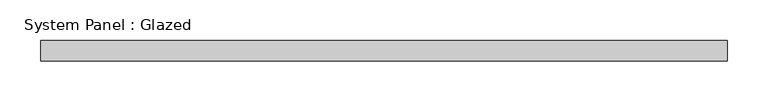
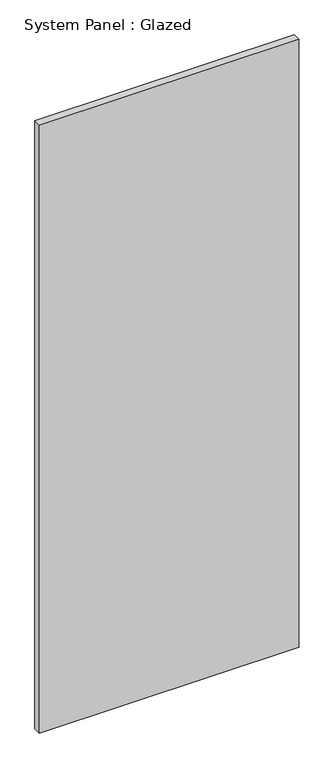
"""IFC4 building model written with IfcOpenShell, lengths in millimetres: plate geometry, System Panel : Glazed."""

from ifc_helpers import new_model, si_unit, origin, origin_with_axes, place, context, project, spatial, polyline, outline, extrude, source, transform, mapped, element, save


def system_panel_glazed_fc786b5a(model_context):
    return source(origin(), model_context, "Body", "SweptSolid", [
        extrude(outline(polyline([(422.275, 19.05), (-422.275, 19.05), (-422.275, 44.45), (422.275, 44.45), (422.275, 19.05)])), origin_with_axes(), (0.0, 0.0, 1.0), 2093.4042846),
    ])


if __name__ == "__main__":
    model = new_model("IFC4")
    model_context = context("Model", 3, world=origin())
    ifc_project = project(units=[si_unit("LENGTHUNIT", "METRE", prefix="MILLI")], contexts=[model_context])
    site = spatial("IfcSite", under=ifc_project)
    building = spatial("IfcBuilding", under=site)
    placement = place(None, origin())
    system_panel_glazed_shape = system_panel_glazed_fc786b5a(model_context)
    element("IfcPlate", 1, ObjectType="System Panel : Glazed", at=placement, inside=building, context=model_context, shape_type="MappedRepresentation", body=[
        mapped(system_panel_glazed_shape, transform((0.0, 0.0, 0.0), x_axis=(1.0, 0.0, 0.0), y_axis=(0.0, 1.0, 0.0), z_axis=(0.0, 0.0, 1.0))),
    ])
    save(model, "model.ifc")

# Revit data of these elements
# Type "System Panel : Glazed"
#   Construction Type Id = "GSP4R"
#   Analytic Construction = "1/8 in Pilkington single glazing"
#   Visual Light Transmittance = 0.9
#   Solar Heat Gain Coefficient = 0.86
#   Heat Transfer Coefficient (U) = 1.18115 BTU/(h·ft²·°F)
#   Define Thermal Properties by = 1
# Element 1 (IfcPlate, "System Panel : Glazed")
#   Materials on its faces: "Glass"
# Materials
#   "Glass": class "Glass", colour RGB 0 128 192, transparency 0.75, Description = "Soda Lime Glass", Cost = 0
